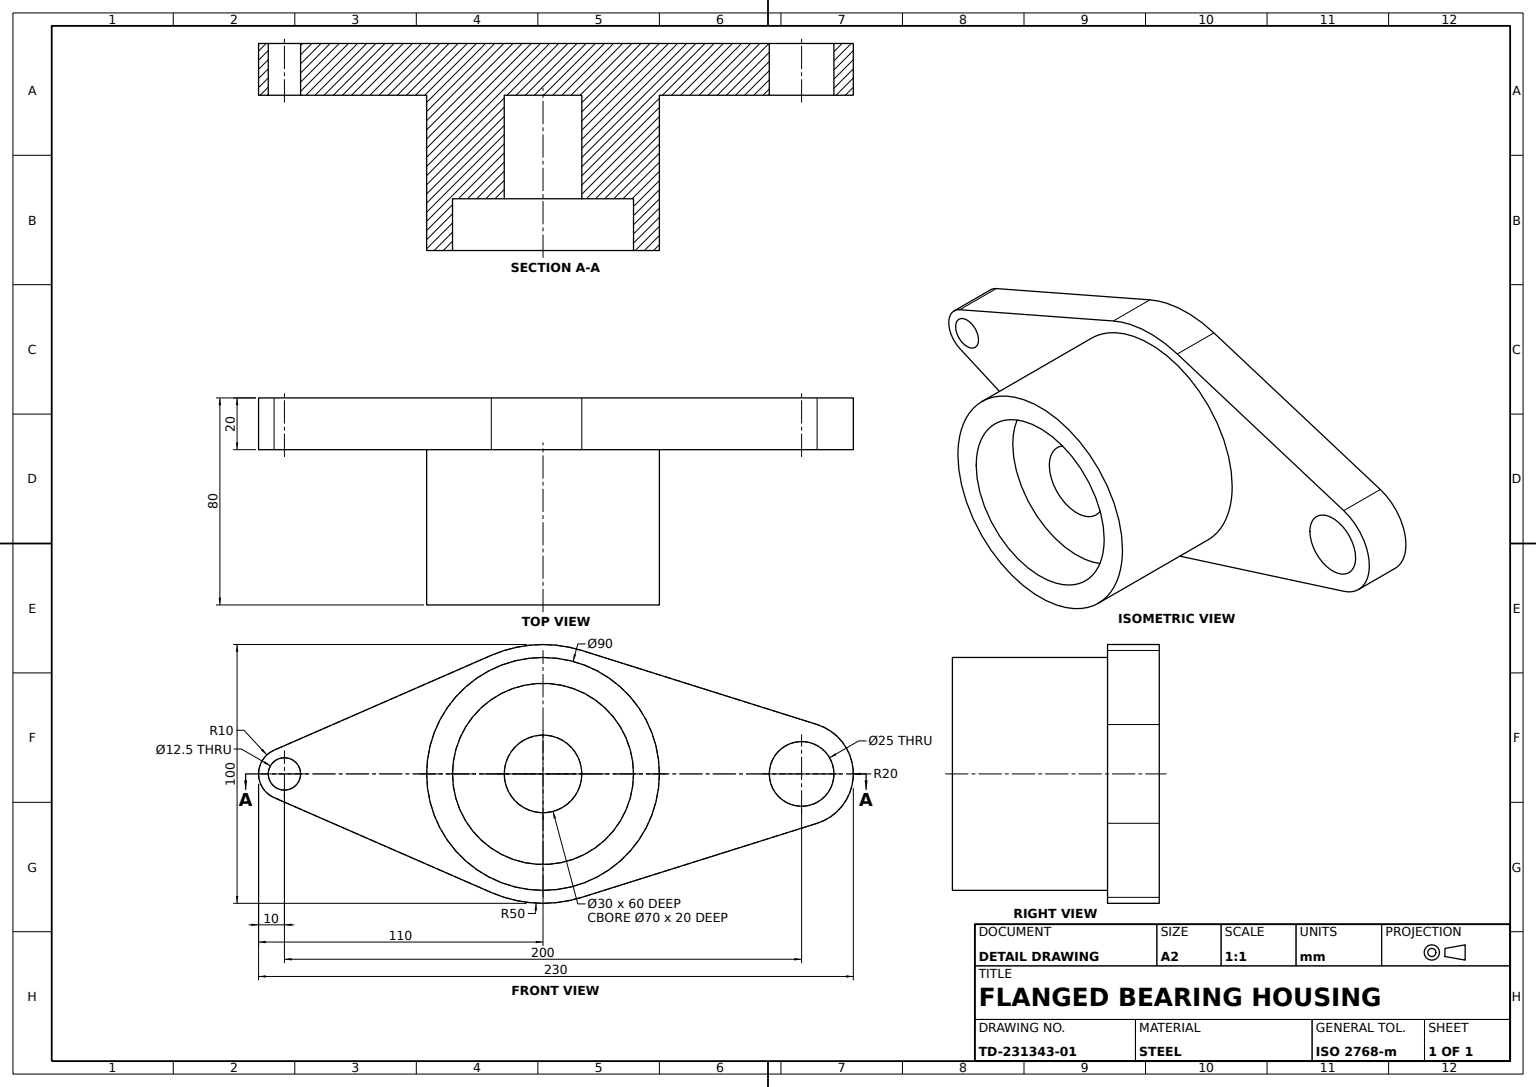
from build123d import *

# Parameters (mm, degrees)
FLANGE_PLATE_PROFILE_R       = 6.25
FLANGE_PLATE_PROFILE_R_2     = 12.5
FLANGE_PLATE_20MM_DEPTH      = 20
HUB_PROFILE_90_70_R          = 45
HUB_PROFILE_90_70_R_2        = 35
HUB_90X60_DEPTH              = 60
INNER_BOSS_PROFILE_70_30_R   = 35
INNER_BOSS_PROFILE_70_30_R_2 = 15
INNER_BOSS_70_BORE_30_DEPTH  = 40


with BuildPart() as part:
    # Flange Plate Profile → Flange Plate 20mm (new body)
    with BuildSketch(Plane.XY):
        with BuildLine():
            Line((-4, 9.16515139), (80, 45.82575695))
            ThreePointArc((80, 45.82575695), (97.330664824, 49.928695654), (115, 47.696960071))
            Line((115, 47.696960071), (206, 19.078784028))
            ThreePointArc((206, 19.078784028), (220, 0), (206, -19.078784028))
            Line((206, -19.078784028), (115, -47.696960071))
            ThreePointArc((115, -47.696960071), (97.330664824, -49.928695654), (80, -45.82575695))
            Line((80, -45.82575695), (-4, -9.16515139))
            ThreePointArc((-4, -9.16515139), (-10, 0), (-4, 9.16515139))
        make_face()
        Circle(FLANGE_PLATE_PROFILE_R, mode=Mode.SUBTRACT)
        with Locations((200, 0)):
            Circle(FLANGE_PLATE_PROFILE_R_2, mode=Mode.SUBTRACT)
    extrude(amount=FLANGE_PLATE_20MM_DEPTH)

    # Hub Profile Ø90-Ø70 → Hub Ø90x60 (add)
    with BuildSketch(Plane.XY.offset(20)):
        with Locations((100, 0)):
            Circle(HUB_PROFILE_90_70_R)
        with Locations((100, 0)):
            Circle(HUB_PROFILE_90_70_R_2, mode=Mode.SUBTRACT)
    extrude(amount=HUB_90X60_DEPTH)

    # Inner Boss Profile Ø70-Ø30 → Inner Boss Ø70 Bore Ø30 (add)
    with BuildSketch(Plane.XY.offset(20)):
        with Locations((100, 0)):
            Circle(INNER_BOSS_PROFILE_70_30_R)
        with Locations((100, 0)):
            Circle(INNER_BOSS_PROFILE_70_30_R_2, mode=Mode.SUBTRACT)
    extrude(amount=INNER_BOSS_70_BORE_30_DEPTH)


solid = part.part
